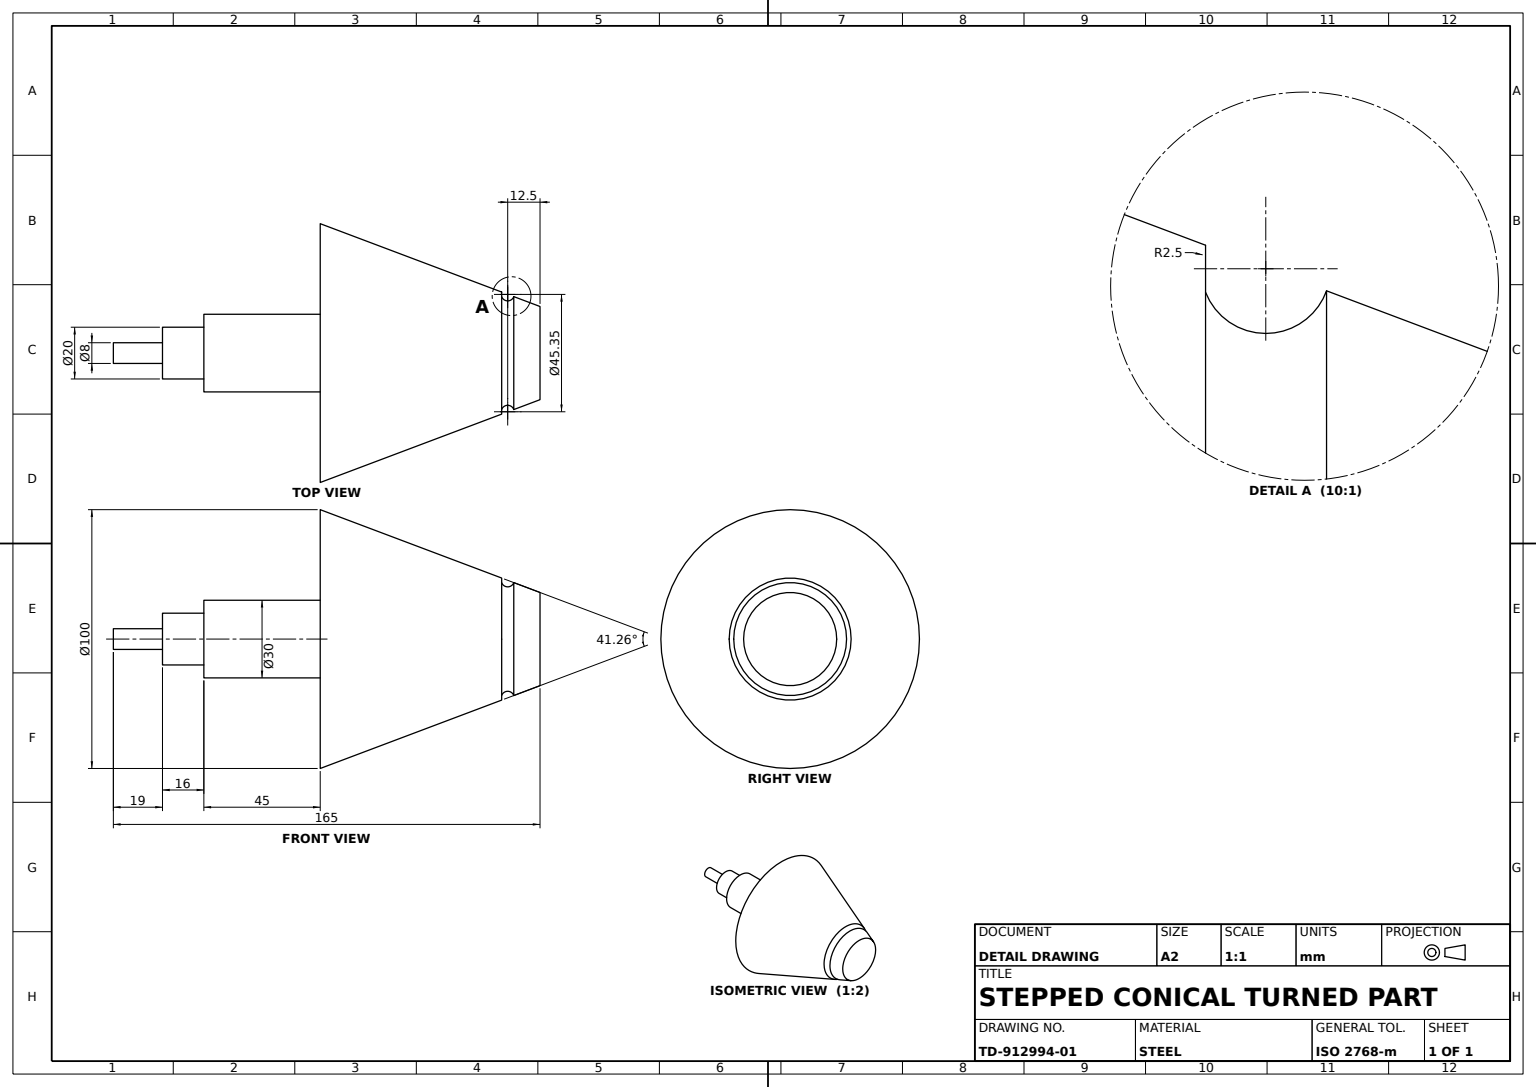
from build123d import *

# Parameters (mm, degrees)
SHAFT_BASE_30_SKETCH_R     = 15
SHAFT_BASE_30_DEPTH        = 45
SHAFT_STEP_2_SKETCH_R      = 10
SHAFT_STEP_2_DEPTH         = 16
SHAFT_TIP_SKETCH_R         = 4
SHAFT_TIP_DEPTH            = 19
CONE_SMALL_END_36_SKETCH_R = 18
CONE_BASE_100_SKETCH_R     = 50
GROOVE_SWEEP_CUT_PROFILE_R = 2.5


with BuildPart() as part:
    # Shaft Base Ø30 Sketch → Shaft Base Ø30 (new body)
    with BuildSketch(Plane.XY):
        with Locations(Location((0, 0, 0), (0, 0, 180))):
            Circle(SHAFT_BASE_30_SKETCH_R)
    extrude(amount=SHAFT_BASE_30_DEPTH)

    # Shaft Step 2 Sketch → Shaft Step 2 (add)
    with BuildSketch(Plane.XY.offset(45)):
        Circle(SHAFT_STEP_2_SKETCH_R)
    extrude(amount=SHAFT_STEP_2_DEPTH)

    # Shaft Tip Sketch → Shaft Tip (add)
    with BuildSketch(Plane.XY.offset(61)):
        Circle(SHAFT_TIP_SKETCH_R)
    extrude(amount=SHAFT_TIP_DEPTH)

    # Cone Small End Ø36 Sketch → Conical Body section 0
    with BuildSketch(Plane(origin=(0, 0, -85), x_dir=(-1, 0, 0), z_dir=(0, 0, -1))):
        Circle(CONE_SMALL_END_36_SKETCH_R)
    # Cone Base Ø100 Sketch → Conical Body section 1
    with BuildSketch(Plane(origin=(0, 0, 0), x_dir=(-1, 0, 0), z_dir=(0, 0, -1))):
        Circle(CONE_BASE_100_SKETCH_R)
    loft()

    # Groove Sweep Cut: sweep along a path in Groove Path
    with BuildLine(Plane(origin=(0, 0, -72.5), x_dir=(-1, 0, 0), z_dir=(0, 0, -1))) as groove_sweep_cut_path:
        CenterArc((0, 0), 22.673462662, 0, 360)
    # Groove Sweep Cut profile (on start of the path) → Groove Sweep Cut (sweep, cut)
    with BuildSketch(Plane(origin=(-22.673462662, 0, -72.5), x_dir=(0, 0, 1), z_dir=(0, 1, 0))):
        Circle(GROOVE_SWEEP_CUT_PROFILE_R)
    sweep(path=groove_sweep_cut_path.line, mode=Mode.SUBTRACT)


solid = part.part
